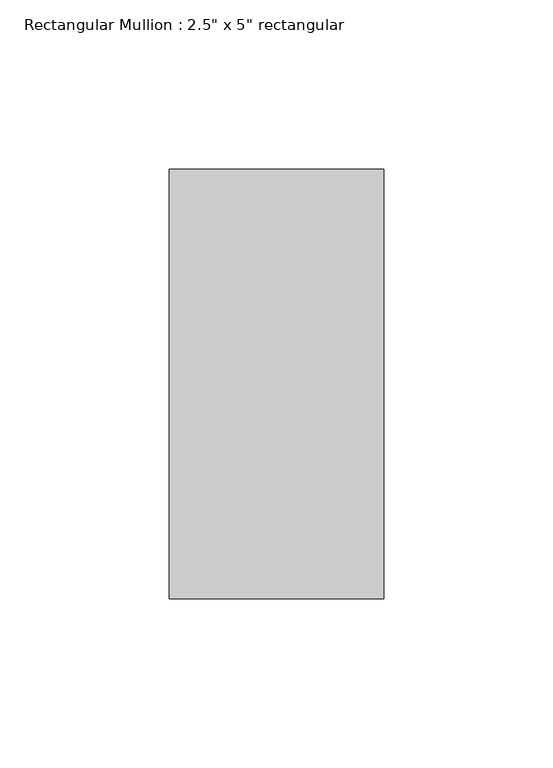
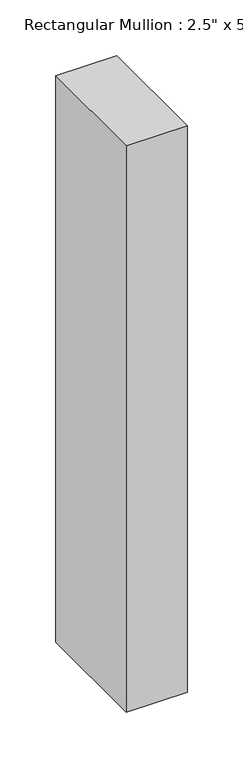
"""IFC4 building model written with IfcOpenShell, lengths in millimetres: member geometry."""

from ifc_helpers import new_model, si_unit, frame, origin, place, context, project, spatial, polyline, outline, extrude, source, transform, mapped, element, save


def member_75a79c70(model_context):
    return source(origin(), model_context, "Body", "SweptSolid", [
        extrude(outline(polyline([(31.75, 63.5), (31.75, -63.5), (-31.75, -63.5), (-31.75, 63.5), (31.75, 63.5)])), frame((0.0, 0.0, -622.3), z_axis=(0.0, 0.0, 1.0), x_axis=(1.0, 0.0, 0.0)), (0.0, 0.0, 1.0), 622.3),
    ])


if __name__ == "__main__":
    model = new_model("IFC4")
    model_context = context("Model", 3, world=origin())
    ifc_project = project(units=[si_unit("LENGTHUNIT", "METRE", prefix="MILLI")], contexts=[model_context])
    site = spatial("IfcSite", under=ifc_project)
    building = spatial("IfcBuilding", under=site)
    placement = place(None, origin())
    member_shape = member_75a79c70(model_context)
    element("IfcMember", 1, ObjectType="Rectangular Mullion : 2.5\" x 5\" rectangular", at=placement, inside=building, context=model_context, shape_type="MappedRepresentation", body=[
        mapped(member_shape, transform((0.0, 0.0, 0.0), x_axis=(1.0, 0.0, 0.0), y_axis=(0.0, 1.0, 0.0), z_axis=(0.0, 0.0, 1.0))),
    ])
    save(model, "model.ifc")

# Revit data of these elements
# Type "Rectangular Mullion : 2.5\" x 5\" rectangular"
#   built-in parameter 1007304 = 0.416667 (stored number, unit not read)
#   built-in parameter 1007301 = 0.104167 (stored number, unit not read)
#   built-in parameter 1007300 = 0.104167 (stored number, unit not read)
# Element 1 (IfcMember, "Rectangular Mullion : 2.5\" x 5\" rectangular")
#   Materials on its faces: "Aluminum"
# Materials
#   "Aluminum": class "Metal", colour RGB 247 247 247, transparency 0, Description = "Aluminum 6061", Cost = 0
